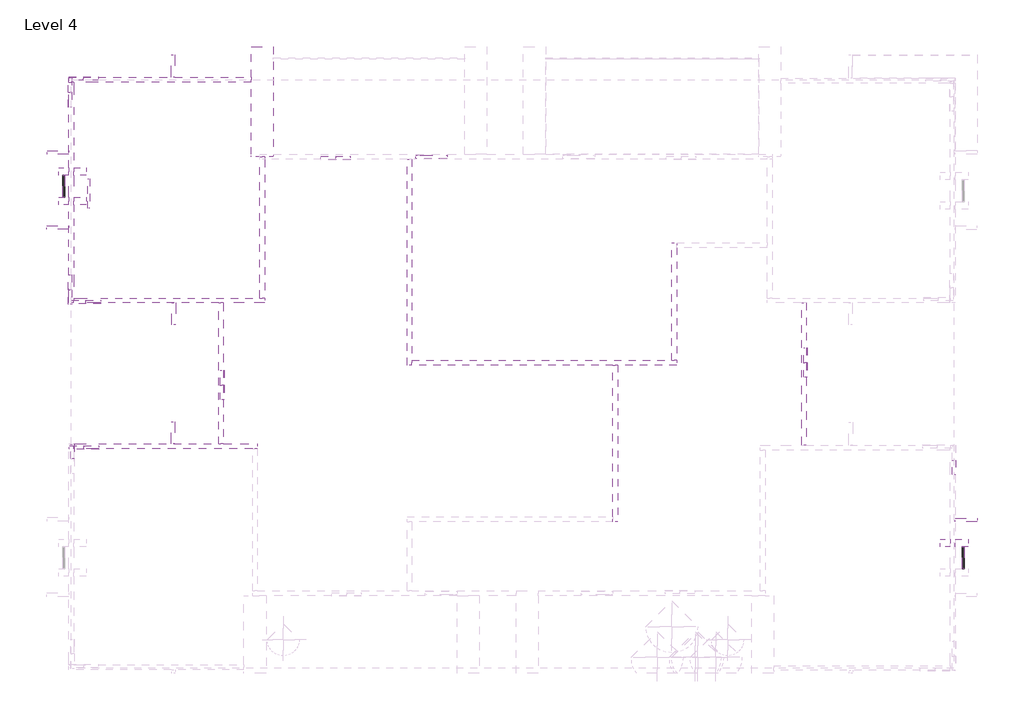
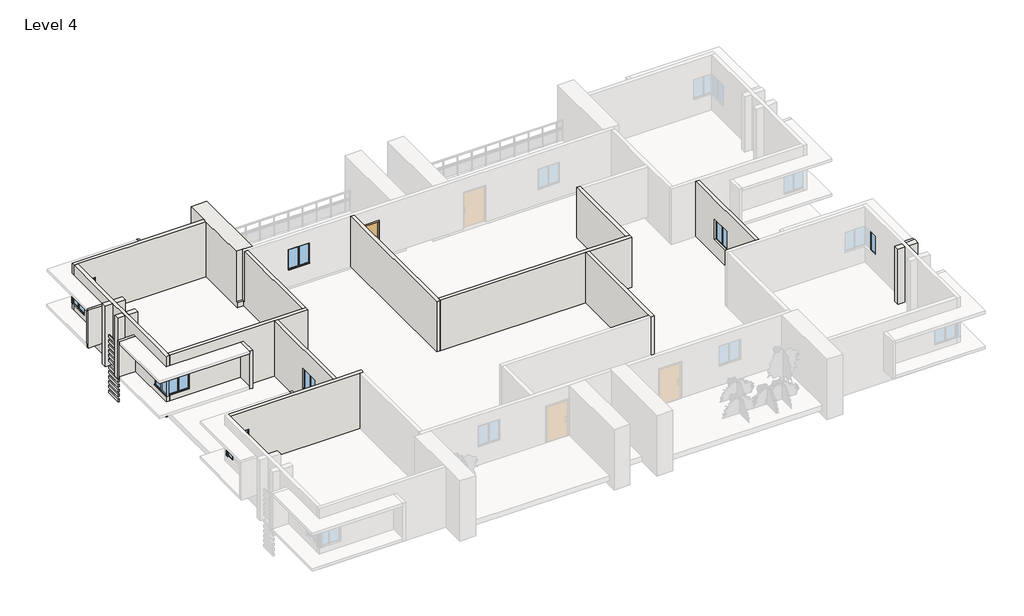
# One storey, part 2 of 4: 49 walls, 18 windows, 1 door.
"""IFC4 building model written with IfcOpenShell, lengths in millimetres."""

from ifc_helpers import new_model, si_unit, frame, origin, place, context, project, spatial, polyline, outline, extrude, faceted_brep, transform, mapped, element, save
from components import door_15d3c954, window_20ff4747

model = new_model("IFC4")

# Units and contexts
model_context = context("Model", 3, world=origin())
ifc_project = project(units=[si_unit("LENGTHUNIT", "METRE", prefix="MILLI")], contexts=[model_context])

# Site, building, storey
site = spatial("IfcSite", under=ifc_project)
building = spatial("IfcBuilding", under=site)
storey = spatial("IfcBuildingStorey", under=building, Name="Level 4", Elevation=9144.0)

# Door
placement = place(None, origin())
door_shape = door_15d3c954(model_context)
element("IfcDoor", 1, ObjectType="Door-Passage-Single-Flush-Dbl_Acting : 48\" x 96\"", at=placement, inside=storey, context=model_context, shape_type="MappedRepresentation", body=[
    mapped(door_shape, transform((153.0520665, 12804.5205944, 10972.8), x_axis=(1.0, 0.0, 0.0), y_axis=(0.0, 1.0, 0.0), z_axis=(0.0, 0.0, 1.0))),
])

# Walls
element("IfcWall", 2, ObjectType="Generic - 1'", at=placement, inside=storey, context=model_context, shape_type="SweptSolid", body=[
    extrude(outline(polyline([(-14151.7972154, 12048.8705944), (-14667.8479335, 12048.8705944), (-14667.8479335, 12353.6705944), (-14151.7972154, 12353.6705944), (-14151.7972154, 12048.8705944)])), frame((0.0, 0.0, 10363.2), z_axis=(0.0, 0.0, 1.0), x_axis=(1.0, 0.0, 0.0)), (0.0, 0.0, 1.0), 3657.6),
])
element("IfcWall", 3, ObjectType="Generic - 1'", at=placement, inside=storey, context=model_context, shape_type="SweptSolid", body=[
    extrude(outline(polyline([(-15302.1394029, 12353.6705944), (-14871.0479335, 12353.6705944), (-14871.0479335, 12048.8705944), (-15302.1394029, 12048.8705944), (-15302.1394029, 12353.6705944)])), frame((0.0, 0.0, 10363.2), z_axis=(0.0, 0.0, 1.0), x_axis=(1.0, 0.0, 0.0)), (0.0, 0.0, 1.0), 3657.6),
])
element("IfcWall", 4, ObjectType="Generic - 1'", at=placement, inside=storey, context=model_context, shape_type="SweptSolid", body=[
    extrude(outline(polyline([(-14151.7972154, 10829.6705944), (-14667.8479335, 10829.6705944), (-14667.8479335, 11134.4705944), (-14151.7972154, 11134.4705944), (-14151.7972154, 10829.6705944)])), frame((0.0, 0.0, 10363.2), z_axis=(0.0, 0.0, 1.0), x_axis=(1.0, 0.0, 0.0)), (0.0, 0.0, 1.0), 3657.6),
])
element("IfcWall", 5, ObjectType="Generic - 1'", at=placement, inside=storey, context=model_context, shape_type="SweptSolid", body=[
    extrude(outline(polyline([(-15302.1394029, 11134.4705944), (-14871.0479335, 11134.4705944), (-14871.0479335, 10829.6705944), (-15302.1394029, 10829.6705944), (-15302.1394029, 11134.4705944)])), frame((0.0, 0.0, 10363.2), z_axis=(0.0, 0.0, 1.0), x_axis=(1.0, 0.0, 0.0)), (0.0, 0.0, 1.0), 3657.6),
])
element("IfcWall", 6, ObjectType="Generic - 1'", at=placement, inside=storey, context=model_context, shape_type="SweptSolid", body=[
    extrude(outline(polyline([(22386.1027846, -3343.5294056), (21857.3520665, -3343.5294056), (21857.3520665, -3038.7294056), (22386.1027846, -3038.7294056), (22386.1027846, -3343.5294056)])), frame((0.0, 0.0, 10363.2), z_axis=(0.0, 0.0, 1.0), x_axis=(1.0, 0.0, 0.0)), (0.0, 0.0, 1.0), 3657.6),
])
element("IfcWall", 7, ObjectType="Generic - 1'", at=placement, inside=storey, context=model_context, shape_type="SweptSolid", body=[
    extrude(outline(polyline([(21235.7605971, -3038.7294056), (21654.1520665, -3038.7294056), (21654.1520665, -3343.5294056), (21235.7605971, -3343.5294056), (21235.7605971, -3038.7294056)])), frame((0.0, 0.0, 10363.2), z_axis=(0.0, 0.0, 1.0), x_axis=(1.0, 0.0, 0.0)), (0.0, 0.0, 1.0), 3657.6),
])
element("IfcWall", 8, ObjectType="Generic - 3'", at=placement, inside=storey, context=model_context, shape_type="Brep", body=[
    faceted_brep([(-6400.1479335, 12810.8705944, 10363.2), (-6400.1479335, 17382.8705944, 10363.2), (-6400.1479335, 17382.8705944, 14020.8), (-6400.1479335, 12912.4705944, 14020.8), (-6400.1479335, 12912.4705944, 10972.8), (-6400.1479335, 12810.8705944, 10972.8), (-7314.5479335, 12810.8705944, 10363.2), (-7314.5479335, 12810.8705944, 10972.8), (-7314.5479335, 12912.4705944, 10972.8), (-7314.5479335, 12912.4705944, 14020.8), (-7314.5479335, 15904.9548886, 14020.8), (-7314.5479335, 16108.1548886, 14020.8), (-7314.5479335, 17382.8705944, 14020.8), (-7314.5479335, 17382.8705944, 10363.2), (-7314.5479335, 16108.1548886, 10363.2), (-7314.5479335, 15904.9548886, 10363.2), (-6755.7479335, 12810.8705944, 10363.2), (-6958.9479335, 12810.8705944, 10363.2), (-6958.9479335, 12912.4705944, 14020.8), (-6755.7479335, 12810.8705944, 10972.8), (-6958.9479335, 12810.8705944, 10972.8), (-6958.9479335, 12912.4705944, 10972.8)], [[[0, 1, 2, 3, 4, 5]], [[6, 7, 8, 9, 10, 11, 12, 13, 14, 15]], [[1, 0, 16, 17, 6, 15, 14, 13]], [[2, 1, 13, 12]], [[3, 2, 12, 11, 10, 9, 18]], [[0, 5, 19, 20, 7, 6, 17, 16]], [[4, 21, 8, 7, 20, 19, 5]], [[4, 3, 18, 9, 8, 21]]]),
])
element("IfcWall", 9, ObjectType="Generic - 5\"", at=placement, inside=storey, context=model_context, shape_type="SweptSolid", body=[
    extrude(outline(polyline([(-15124.6936682, 11134.4705944), (-15124.6936682, 12048.8705944), (-15048.4936682, 12048.8705944), (-15048.4936682, 11134.4705944), (-15124.6936682, 11134.4705944)])), frame((0.0, 0.0, 8712.2), z_axis=(0.0, 0.0, 1.0), x_axis=(1.0, 0.0, 0.0)), (0.0, 0.0, 1.0), 152.8735856),
])
element("IfcWall", 10, ObjectType="Generic - 5\"", at=placement, inside=storey, context=model_context, shape_type="SweptSolid", body=[
    extrude(outline(polyline([(-15124.6936682, 11134.4705944), (-15124.6936682, 12048.8705944), (-15048.4936682, 12048.8705944), (-15048.4936682, 11134.4705944), (-15124.6936682, 11134.4705944)])), frame((0.0, 0.0, 9017.0), z_axis=(0.0, 0.0, 1.0), x_axis=(1.0, 0.0, 0.0)), (0.0, 0.0, 1.0), 152.8735856),
])
element("IfcWall", 11, ObjectType="Generic - 5\"", at=placement, inside=storey, context=model_context, shape_type="SweptSolid", body=[
    extrude(outline(polyline([(-15124.6936682, 11134.4705944), (-15124.6936682, 12048.8705944), (-15048.4936682, 12048.8705944), (-15048.4936682, 11134.4705944), (-15124.6936682, 11134.4705944)])), frame((0.0, 0.0, 9296.4), z_axis=(0.0, 0.0, 1.0), x_axis=(1.0, 0.0, 0.0)), (0.0, 0.0, 1.0), 152.8735856),
])
element("IfcWall", 12, ObjectType="Generic - 5\"", at=placement, inside=storey, context=model_context, shape_type="SweptSolid", body=[
    extrude(outline(polyline([(-15124.6936682, 11134.4705944), (-15124.6936682, 12048.8705944), (-15048.4936682, 12048.8705944), (-15048.4936682, 11134.4705944), (-15124.6936682, 11134.4705944)])), frame((0.0, 0.0, 9601.2), z_axis=(0.0, 0.0, 1.0), x_axis=(1.0, 0.0, 0.0)), (0.0, 0.0, 1.0), 152.8735856),
])
element("IfcWall", 13, ObjectType="Generic - 5\"", at=placement, inside=storey, context=model_context, shape_type="SweptSolid", body=[
    extrude(outline(polyline([(-15124.6936682, 11134.4705944), (-15124.6936682, 12048.8705944), (-15048.4936682, 12048.8705944), (-15048.4936682, 11134.4705944), (-15124.6936682, 11134.4705944)])), frame((0.0, 0.0, 9906.0), z_axis=(0.0, 0.0, 1.0), x_axis=(1.0, 0.0, 0.0)), (0.0, 0.0, 1.0), 152.8735856),
])
element("IfcWall", 14, ObjectType="Generic - 5\"", at=placement, inside=storey, context=model_context, shape_type="SweptSolid", body=[
    extrude(outline(polyline([(-15124.6936682, 11134.4705944), (-15124.6936682, 12048.8705944), (-15048.4936682, 12048.8705944), (-15048.4936682, 11134.4705944), (-15124.6936682, 11134.4705944)])), frame((0.0, 0.0, 10210.8), z_axis=(0.0, 0.0, 1.0), x_axis=(1.0, 0.0, 0.0)), (0.0, 0.0, 1.0), 152.8735856),
])
element("IfcWall", 15, ObjectType="Generic - 5\"", at=placement, inside=storey, context=model_context, shape_type="SweptSolid", body=[
    extrude(outline(polyline([(22145.9857703, -4257.9294056), (22145.9857703, -3343.5294056), (22222.1857703, -3343.5294056), (22222.1857703, -4257.9294056), (22145.9857703, -4257.9294056)])), frame((0.0, 0.0, 8712.2), z_axis=(0.0, 0.0, 1.0), x_axis=(1.0, 0.0, 0.0)), (0.0, 0.0, 1.0), 152.8735856),
])
element("IfcWall", 16, ObjectType="Generic - 5\"", at=placement, inside=storey, context=model_context, shape_type="SweptSolid", body=[
    extrude(outline(polyline([(22145.9857703, -4257.9294056), (22145.9857703, -3343.5294056), (22222.1857703, -3343.5294056), (22222.1857703, -4257.9294056), (22145.9857703, -4257.9294056)])), frame((0.0, 0.0, 9017.0), z_axis=(0.0, 0.0, 1.0), x_axis=(1.0, 0.0, 0.0)), (0.0, 0.0, 1.0), 152.8735856),
])
element("IfcWall", 17, ObjectType="Generic - 5\"", at=placement, inside=storey, context=model_context, shape_type="SweptSolid", body=[
    extrude(outline(polyline([(22145.9857703, -4257.9294056), (22145.9857703, -3343.5294056), (22222.1857703, -3343.5294056), (22222.1857703, -4257.9294056), (22145.9857703, -4257.9294056)])), frame((0.0, 0.0, 9296.4), z_axis=(0.0, 0.0, 1.0), x_axis=(1.0, 0.0, 0.0)), (0.0, 0.0, 1.0), 152.8735856),
])
element("IfcWall", 18, ObjectType="Generic - 5\"", at=placement, inside=storey, context=model_context, shape_type="SweptSolid", body=[
    extrude(outline(polyline([(22145.9857703, -4257.9294056), (22145.9857703, -3343.5294056), (22222.1857703, -3343.5294056), (22222.1857703, -4257.9294056), (22145.9857703, -4257.9294056)])), frame((0.0, 0.0, 9601.2), z_axis=(0.0, 0.0, 1.0), x_axis=(1.0, 0.0, 0.0)), (0.0, 0.0, 1.0), 152.8735856),
])
element("IfcWall", 19, ObjectType="Generic - 5\"", at=placement, inside=storey, context=model_context, shape_type="SweptSolid", body=[
    extrude(outline(polyline([(22145.9857703, -4257.9294056), (22145.9857703, -3343.5294056), (22222.1857703, -3343.5294056), (22222.1857703, -4257.9294056), (22145.9857703, -4257.9294056)])), frame((0.0, 0.0, 9906.0), z_axis=(0.0, 0.0, 1.0), x_axis=(1.0, 0.0, 0.0)), (0.0, 0.0, 1.0), 152.8735856),
])
element("IfcWall", 20, ObjectType="Generic - 5\"", at=placement, inside=storey, context=model_context, shape_type="SweptSolid", body=[
    extrude(outline(polyline([(22145.9857703, -4257.9294056), (22145.9857703, -3343.5294056), (22222.1857703, -3343.5294056), (22222.1857703, -4257.9294056), (22145.9857703, -4257.9294056)])), frame((0.0, 0.0, 10210.8), z_axis=(0.0, 0.0, 1.0), x_axis=(1.0, 0.0, 0.0)), (0.0, 0.0, 1.0), 152.8735856),
])
element("IfcWall", 21, ObjectType="Generic - 5\"", at=placement, inside=storey, context=model_context, shape_type="SweptSolid", body=[
    extrude(outline(polyline([(-15124.6936682, 11134.4705944), (-15124.6936682, 12048.8705944), (-15048.4936682, 12048.8705944), (-15048.4936682, 11134.4705944), (-15124.6936682, 11134.4705944)])), frame((0.0, 0.0, 10617.2), z_axis=(0.0, 0.0, 1.0), x_axis=(1.0, 0.0, 0.0)), (0.0, 0.0, 1.0), 152.8735856),
])
element("IfcWall", 22, ObjectType="Generic - 5\"", at=placement, inside=storey, context=model_context, shape_type="SweptSolid", body=[
    extrude(outline(polyline([(-14084.4224108, 10677.2705944), (-14084.4224108, 11896.4705944), (-14008.2224108, 11896.4705944), (-14008.2224108, 10677.2705944), (-14084.4224108, 10677.2705944)])), frame((0.0, 0.0, 10617.2), z_axis=(0.0, 0.0, 1.0), x_axis=(1.0, 0.0, 0.0)), (0.0, 0.0, 1.0), 178.1810075),
])
element("IfcWall", 23, ObjectType="Generic - 5\"", at=placement, inside=storey, context=model_context, shape_type="SweptSolid", body=[
    extrude(outline(polyline([(-15124.6936682, 11134.4705944), (-15124.6936682, 12048.8705944), (-15048.4936682, 12048.8705944), (-15048.4936682, 11134.4705944), (-15124.6936682, 11134.4705944)])), frame((0.0, 0.0, 10896.6), z_axis=(0.0, 0.0, 1.0), x_axis=(1.0, 0.0, 0.0)), (0.0, 0.0, 1.0), 152.8735856),
])
element("IfcWall", 24, ObjectType="Generic - 5\"", at=placement, inside=storey, context=model_context, shape_type="SweptSolid", body=[
    extrude(outline(polyline([(-15124.6936682, 11134.4705944), (-15124.6936682, 12048.8705944), (-15048.4936682, 12048.8705944), (-15048.4936682, 11134.4705944), (-15124.6936682, 11134.4705944)])), frame((0.0, 0.0, 11176.0), z_axis=(0.0, 0.0, 1.0), x_axis=(1.0, 0.0, 0.0)), (0.0, 0.0, 1.0), 152.8735856),
])
element("IfcWall", 25, ObjectType="Generic - 5\"", at=placement, inside=storey, context=model_context, shape_type="SweptSolid", body=[
    extrude(outline(polyline([(-15124.6936682, 11134.4705944), (-15124.6936682, 12048.8705944), (-15048.4936682, 12048.8705944), (-15048.4936682, 11134.4705944), (-15124.6936682, 11134.4705944)])), frame((0.0, 0.0, 11480.8), z_axis=(0.0, 0.0, 1.0), x_axis=(1.0, 0.0, 0.0)), (0.0, 0.0, 1.0), 152.8735856),
])
element("IfcWall", 26, ObjectType="Generic - 5\"", at=placement, inside=storey, context=model_context, shape_type="SweptSolid", body=[
    extrude(outline(polyline([(-15124.6936682, 11134.4705944), (-15124.6936682, 12048.8705944), (-15048.4936682, 12048.8705944), (-15048.4936682, 11134.4705944), (-15124.6936682, 11134.4705944)])), frame((0.0, 0.0, 11785.6), z_axis=(0.0, 0.0, 1.0), x_axis=(1.0, 0.0, 0.0)), (0.0, 0.0, 1.0), 152.8735856),
])
element("IfcWall", 27, ObjectType="Generic - 5\"", at=placement, inside=storey, context=model_context, shape_type="SweptSolid", body=[
    extrude(outline(polyline([(-15124.6936682, 11134.4705944), (-15124.6936682, 12048.8705944), (-15048.4936682, 12048.8705944), (-15048.4936682, 11134.4705944), (-15124.6936682, 11134.4705944)])), frame((0.0, 0.0, 12065.0), z_axis=(0.0, 0.0, 1.0), x_axis=(1.0, 0.0, 0.0)), (0.0, 0.0, 1.0), 152.8735856),
])
element("IfcWall", 28, ObjectType="Generic - 5\"", at=placement, inside=storey, context=model_context, shape_type="SweptSolid", body=[
    extrude(outline(polyline([(22145.9857703, -4257.9294056), (22145.9857703, -3343.5294056), (22222.1857703, -3343.5294056), (22222.1857703, -4257.9294056), (22145.9857703, -4257.9294056)])), frame((0.0, 0.0, 10617.2), z_axis=(0.0, 0.0, 1.0), x_axis=(1.0, 0.0, 0.0)), (0.0, 0.0, 1.0), 152.8735856),
])
element("IfcWall", 29, ObjectType="Generic - 5\"", at=placement, inside=storey, context=model_context, shape_type="SweptSolid", body=[
    extrude(outline(polyline([(22145.9857703, -4257.9294056), (22145.9857703, -3343.5294056), (22222.1857703, -3343.5294056), (22222.1857703, -4257.9294056), (22145.9857703, -4257.9294056)])), frame((0.0, 0.0, 10896.6), z_axis=(0.0, 0.0, 1.0), x_axis=(1.0, 0.0, 0.0)), (0.0, 0.0, 1.0), 152.8735856),
])
element("IfcWall", 30, ObjectType="Generic - 5\"", at=placement, inside=storey, context=model_context, shape_type="SweptSolid", body=[
    extrude(outline(polyline([(22145.9857703, -4257.9294056), (22145.9857703, -3343.5294056), (22222.1857703, -3343.5294056), (22222.1857703, -4257.9294056), (22145.9857703, -4257.9294056)])), frame((0.0, 0.0, 11176.0), z_axis=(0.0, 0.0, 1.0), x_axis=(1.0, 0.0, 0.0)), (0.0, 0.0, 1.0), 152.8735856),
])
element("IfcWall", 31, ObjectType="Generic - 5\"", at=placement, inside=storey, context=model_context, shape_type="SweptSolid", body=[
    extrude(outline(polyline([(22145.9857703, -4257.9294056), (22145.9857703, -3343.5294056), (22222.1857703, -3343.5294056), (22222.1857703, -4257.9294056), (22145.9857703, -4257.9294056)])), frame((0.0, 0.0, 11480.8), z_axis=(0.0, 0.0, 1.0), x_axis=(1.0, 0.0, 0.0)), (0.0, 0.0, 1.0), 152.8735856),
])
element("IfcWall", 32, ObjectType="Generic - 5\"", at=placement, inside=storey, context=model_context, shape_type="SweptSolid", body=[
    extrude(outline(polyline([(22145.9857703, -4257.9294056), (22145.9857703, -3343.5294056), (22222.1857703, -3343.5294056), (22222.1857703, -4257.9294056), (22145.9857703, -4257.9294056)])), frame((0.0, 0.0, 11785.6), z_axis=(0.0, 0.0, 1.0), x_axis=(1.0, 0.0, 0.0)), (0.0, 0.0, 1.0), 152.8735856),
])
element("IfcWall", 33, ObjectType="Generic - 5\"", at=placement, inside=storey, context=model_context, shape_type="SweptSolid", body=[
    extrude(outline(polyline([(22145.9857703, -4257.9294056), (22145.9857703, -3343.5294056), (22222.1857703, -3343.5294056), (22222.1857703, -4257.9294056), (22145.9857703, -4257.9294056)])), frame((0.0, 0.0, 12065.0), z_axis=(0.0, 0.0, 1.0), x_axis=(1.0, 0.0, 0.0)), (0.0, 0.0, 1.0), 152.8735856),
])
element("IfcWall", 34, ObjectType="Generic - 6\"", at=placement, inside=storey, context=model_context, shape_type="SweptSolid", body=[
    extrude(outline(polyline([(-10480.7034654, 17035.2548886), (-10480.7034654, 16120.8548886), (-10633.1034654, 16120.8548886), (-10633.1034654, 17035.2548886), (-10480.7034654, 17035.2548886)])), frame((0.0, 0.0, 11125.2), z_axis=(0.0, 0.0, 1.0), x_axis=(1.0, 0.0, 0.0)), (0.0, 0.0, 1.0), 2286.0),
])
element("IfcWall", 35, ObjectType="Generic - 6\"", at=placement, inside=storey, context=model_context, shape_type="SweptSolid", body=[
    extrude(outline(polyline([(-15775.8097154, 13072.8548886), (-14883.7479335, 13072.8548886), (-14883.7479335, 12920.4548886), (-15775.8097154, 12920.4548886), (-15775.8097154, 13072.8548886)])), frame((0.0, 0.0, 11125.2), z_axis=(0.0, 0.0, 1.0), x_axis=(1.0, 0.0, 0.0)), (0.0, 0.0, 1.0), 2286.0),
])
element("IfcWall", 36, ObjectType="Generic - 6\"", at=placement, inside=storey, context=model_context, shape_type="SweptSolid", body=[
    extrude(outline(polyline([(-10603.8479335, 5846.5548886), (-10603.8479335, 6760.9548886), (-10451.4479335, 6760.9548886), (-10451.4479335, 5846.5548886), (-10603.8479335, 5846.5548886)])), frame((0.0, 0.0, 11125.2), z_axis=(0.0, 0.0, 1.0), x_axis=(1.0, 0.0, 0.0)), (0.0, 0.0, 1.0), 2286.0),
])
element("IfcWall", 37, ObjectType="Generic - 6\"", at=placement, inside=storey, context=model_context, shape_type="SweptSolid", body=[
    extrude(outline(polyline([(-15798.1479335, 9961.3548886), (-14883.7479335, 9961.3548886), (-14883.7479335, 9808.9548886), (-15798.1479335, 9808.9548886), (-15798.1479335, 9961.3548886)])), frame((0.0, 0.0, 11125.2), z_axis=(0.0, 0.0, 1.0), x_axis=(1.0, 0.0, 0.0)), (0.0, 0.0, 1.0), 2286.0),
])
element("IfcWall", 38, ObjectType="Generic - 6\"", at=placement, inside=storey, context=model_context, shape_type="SweptSolid", body=[
    extrude(outline(polyline([(-10480.7034654, 1834.0395301), (-10480.7034654, 919.6395301), (-10633.1034654, 919.6395301), (-10633.1034654, 1834.0395301), (-10480.7034654, 1834.0395301)])), frame((0.0, 0.0, 11125.2), z_axis=(0.0, 0.0, 1.0), x_axis=(1.0, 0.0, 0.0)), (0.0, 0.0, 1.0), 2286.0),
])
element("IfcWall", 39, ObjectType="Generic - 6\"", at=placement, inside=storey, context=model_context, shape_type="SweptSolid", body=[
    extrude(outline(polyline([(22771.7520665, -2309.5899195), (21857.3520665, -2309.5899195), (21857.3520665, -2157.1899195), (22771.7520665, -2157.1899195), (22771.7520665, -2309.5899195)])), frame((0.0, 0.0, 11125.2), z_axis=(0.0, 0.0, 1.0), x_axis=(1.0, 0.0, 0.0)), (0.0, 0.0, 1.0), 2286.0),
])
element("IfcWall", 40, ObjectType="Generic - 8\"", at=placement, inside=storey, context=model_context, shape_type="Brep", body=[
    faceted_brep([(-862.9479335, 12709.2705944, 10972.8), (-862.9479335, 4174.8705944, 10972.8), (-862.9479335, 4174.8705944, 14020.8), (-862.9479335, 12709.2705944, 14020.8), (-659.7479335, 12709.2705944, 10972.8), (-659.7479335, 12709.2705944, 14020.8), (-659.7479335, 4378.0705944, 14020.8), (-659.7479335, 4174.8705944, 14020.8), (-659.7479335, 4174.8705944, 10972.8), (-659.7479335, 4378.0705944, 10972.8)], [[[0, 1, 2, 3]], [[4, 5, 6, 7, 8, 9]], [[1, 0, 4, 9, 8]], [[3, 2, 7, 6, 5]], [[0, 3, 5, 4]], [[2, 1, 8, 7]]]),
])
element("IfcWall", 41, ObjectType="Generic - 8\"", at=placement, inside=storey, context=model_context, shape_type="Brep", body=[
    faceted_brep([(-659.7479335, 4174.8705944, 10972.8), (7671.4520665, 4174.8705944, 10972.8), (7874.6520665, 4174.8705944, 10972.8), (10313.0520665, 4174.8705944, 10972.8), (10313.0520665, 4174.8705944, 14020.8), (7874.6520665, 4174.8705944, 14020.8), (7671.4520665, 4174.8705944, 14020.8), (-659.7479335, 4174.8705944, 14020.8), (-659.7479335, 4378.0705944, 10972.8), (-659.7479335, 4378.0705944, 14020.8), (10109.8520665, 4378.0705944, 14020.8), (10313.0520665, 4378.0705944, 14020.8), (10313.0520665, 4378.0705944, 10972.8), (10109.8520665, 4378.0705944, 10972.8)], [[[0, 1, 2, 3, 4, 5, 6, 7]], [[8, 9, 10, 11, 12, 13]], [[3, 2, 1, 0, 8, 13, 12]], [[7, 6, 5, 4, 11, 10, 9]], [[0, 7, 9, 8]], [[4, 3, 12, 11]]]),
])
element("IfcWall", 42, ObjectType="Generic - 8\"", at=placement, inside=storey, context=model_context, shape_type="Brep", body=[
    faceted_brep([(10313.0520665, 4378.0705944, 10972.8), (10313.0520665, 9051.6705944, 10972.8), (10313.0520665, 9254.8705944, 10972.8), (10313.0520665, 9254.8705944, 14020.8), (10313.0520665, 9051.6705944, 14020.8), (10313.0520665, 4378.0705944, 14020.8), (10109.8520665, 4378.0705944, 10972.8), (10109.8520665, 4378.0705944, 14020.8), (10109.8520665, 9254.8705944, 14020.8), (10109.8520665, 9254.8705944, 10972.8)], [[[0, 1, 2, 3, 4, 5]], [[6, 7, 8, 9]], [[2, 1, 0, 6, 9]], [[5, 4, 3, 8, 7]], [[0, 5, 7, 6]], [[3, 2, 9, 8]]]),
])
element("IfcWall", 43, ObjectType="Generic - 8\"", at=placement, inside=storey, context=model_context, shape_type="Brep", body=[
    faceted_brep([(7671.4520665, 4174.8705944, 10972.8), (7671.4520665, -2102.9604699, 10972.8), (7671.4520665, -2306.1604699, 10972.8), (7671.4520665, -2306.1604699, 14020.8), (7671.4520665, -2102.9604699, 14020.8), (7671.4520665, 4174.8705944, 14020.8), (7874.6520665, 4174.8705944, 10972.8), (7874.6520665, 4174.8705944, 14020.8), (7874.6520665, -2306.1604699, 14020.8), (7874.6520665, -2306.1604699, 10972.8)], [[[0, 1, 2, 3, 4, 5]], [[6, 7, 8, 9]], [[2, 1, 0, 6, 9]], [[5, 4, 3, 8, 7]], [[0, 5, 7, 6]], [[3, 2, 9, 8]]]),
])
element("IfcWall", 44, ObjectType="Generic - 8\" gray", at=placement, inside=storey, context=model_context, shape_type="Brep", body=[
    faceted_brep([(-14871.0479335, 15904.9548886, 10363.2), (-14667.8479335, 15904.9548886, 10363.2), (-7314.5479335, 15904.9548886, 10363.2), (-7314.5479335, 15904.9548886, 14020.8), (-14667.8479335, 15904.9548886, 14020.8), (-14871.0479335, 15904.9548886, 14020.8), (-14871.0479335, 15904.9548886, 12854.6804451), (-14667.8479335, 15904.9548886, 12854.6804451), (-13661.292575, 15904.9548886, 12854.6804451), (-13661.292575, 15904.9548886, 11635.4804451), (-14667.8479335, 15904.9548886, 11635.4804451), (-14871.0479335, 15904.9548886, 11635.4804451), (-7314.5479335, 16108.1548886, 10363.2), (-14871.0479335, 16108.1548886, 10363.2), (-14871.0479335, 16108.1548886, 11635.4804451), (-13661.292575, 16108.1548886, 11635.4804451), (-13661.292575, 16108.1548886, 12854.6804451), (-14871.0479335, 16108.1548886, 12854.6804451), (-14871.0479335, 16108.1548886, 14020.8), (-7314.5479335, 16108.1548886, 14020.8)], [[[0, 1, 2, 3, 4, 5, 6, 7, 8, 9, 10, 11]], [[12, 13, 14, 15, 16, 17, 18, 19]], [[2, 1, 0, 13, 12]], [[5, 4, 3, 19, 18]], [[5, 18, 17, 6]], [[13, 0, 11, 14]], [[3, 2, 12, 19]], [[9, 15, 14, 11, 10]], [[6, 17, 16, 8, 7]], [[8, 16, 15, 9]]]),
])
element("IfcWall", 45, ObjectType="Generic - 8\" gray", at=placement, inside=storey, context=model_context, shape_type="Brep", body=[
    faceted_brep([(-14667.8479335, 6760.9548886, 10363.2), (-14667.8479335, 6964.1548886, 10363.2), (-14667.8479335, 10829.6705944, 10363.2), (-14667.8479335, 11134.4705944, 10363.2), (-14667.8479335, 12048.8705944, 10363.2), (-14667.8479335, 12353.6705944, 10363.2), (-14667.8479335, 15904.9548886, 10363.2), (-14667.8479335, 15904.9548886, 11635.4804451), (-14667.8479335, 14871.0236266, 11635.4804451), (-14667.8479335, 14871.0236266, 12854.6804451), (-14667.8479335, 15904.9548886, 12854.6804451), (-14667.8479335, 15904.9548886, 14020.8), (-14667.8479335, 12353.6705944, 14020.8), (-14667.8479335, 12048.8705944, 14020.8), (-14667.8479335, 11134.4705944, 14020.8), (-14667.8479335, 10829.6705944, 14020.8), (-14667.8479335, 6964.1548886, 14020.8), (-14667.8479335, 6760.9548886, 14020.8), (-14667.8479335, 6760.9548886, 12854.6804451), (-14667.8479335, 6964.1548886, 12854.6804451), (-14667.8479335, 7918.4820466, 12854.6804451), (-14667.8479335, 7918.4820466, 11635.4804451), (-14667.8479335, 6964.1548886, 11635.4804451), (-14667.8479335, 6760.9548886, 11635.4804451), (-14871.0479335, 15904.9548886, 10363.2), (-14871.0479335, 12353.6705944, 10363.2), (-14871.0479335, 12048.8705944, 10363.2), (-14871.0479335, 11134.4705944, 10363.2), (-14871.0479335, 10829.6705944, 10363.2), (-14871.0479335, 6760.9548886, 10363.2), (-14871.0479335, 6760.9548886, 11635.4804451), (-14871.0479335, 7918.4820466, 11635.4804451), (-14871.0479335, 7918.4820466, 12854.6804451), (-14871.0479335, 6760.9548886, 12854.6804451), (-14871.0479335, 6760.9548886, 14020.8), (-14871.0479335, 10829.6705944, 14020.8), (-14871.0479335, 11134.4705944, 14020.8), (-14871.0479335, 12048.8705944, 14020.8), (-14871.0479335, 12353.6705944, 14020.8), (-14871.0479335, 15904.9548886, 14020.8), (-14871.0479335, 15904.9548886, 12854.6804451), (-14871.0479335, 14871.0236266, 12854.6804451), (-14871.0479335, 14871.0236266, 11635.4804451), (-14871.0479335, 15904.9548886, 11635.4804451)], [[[0, 1, 2, 3, 4, 5, 6, 7, 8, 9, 10, 11, 12, 13, 14, 15, 16, 17, 18, 19, 20, 21, 22, 23]], [[24, 25, 26, 27, 28, 29, 30, 31, 32, 33, 34, 35, 36, 37, 38, 39, 40, 41, 42, 43]], [[6, 5, 4, 3, 2, 1, 0, 29, 28, 27, 26, 25, 24]], [[17, 16, 15, 14, 13, 12, 11, 39, 38, 37, 36, 35, 34]], [[17, 34, 33, 18]], [[29, 0, 23, 30]], [[6, 24, 43, 7]], [[39, 11, 10, 40]], [[30, 23, 22, 21, 31]], [[18, 33, 32, 20, 19]], [[20, 32, 31, 21]], [[7, 43, 42, 8]], [[9, 8, 42, 41]], [[9, 41, 40, 10]]]),
])
element("IfcWall", 46, ObjectType="Generic - 8\" gray", at=placement, inside=storey, context=model_context, shape_type="Brep", body=[
    faceted_brep([(-6755.7479335, 6964.1548886, 10363.2), (-6958.9479335, 6964.1548886, 10363.2), (-14667.8479335, 6964.1548886, 10363.2), (-14667.8479335, 6964.1548886, 11635.4804451), (-13556.3228261, 6964.1548886, 11635.4804451), (-13556.3228261, 6964.1548886, 12854.6804451), (-14667.8479335, 6964.1548886, 12854.6804451), (-14667.8479335, 6964.1548886, 14020.8), (-6958.9479335, 6964.1548886, 14020.8), (-6755.7479335, 6964.1548886, 14020.8), (-14667.8479335, 6760.9548886, 10363.2), (-8673.4479335, 6760.9548886, 10363.2), (-8470.2479335, 6760.9548886, 10363.2), (-6755.7479335, 6760.9548886, 10363.2), (-6755.7479335, 6760.9548886, 14020.8), (-8470.2479335, 6760.9548886, 14020.8), (-8673.4479335, 6760.9548886, 14020.8), (-14667.8479335, 6760.9548886, 14020.8), (-14667.8479335, 6760.9548886, 12854.6804451), (-13556.3228261, 6760.9548886, 12854.6804451), (-13556.3228261, 6760.9548886, 11635.4804451), (-14667.8479335, 6760.9548886, 11635.4804451)], [[[0, 1, 2, 3, 4, 5, 6, 7, 8, 9]], [[10, 11, 12, 13, 14, 15, 16, 17, 18, 19, 20, 21]], [[2, 1, 0, 13, 12, 11, 10]], [[9, 8, 7, 17, 16, 15, 14]], [[2, 10, 21, 3]], [[17, 7, 6, 18]], [[0, 9, 14, 13]], [[3, 21, 20, 4]], [[5, 4, 20, 19]], [[5, 19, 18, 6]]]),
])
element("IfcWall", 47, ObjectType="Generic - 8\" gray", at=placement, inside=storey, context=model_context, shape_type="Brep", body=[
    faceted_brep([(-7060.5479335, 919.6395301, 10363.2), (-8470.2479335, 919.6395301, 10363.2), (-8673.4479335, 919.6395301, 10363.2), (-14680.5479335, 919.6395301, 10363.2), (-14680.5479335, 919.6395301, 11635.4804451), (-13641.9760869, 919.6395301, 11635.4804451), (-13641.9760869, 919.6395301, 12854.6804451), (-14680.5479335, 919.6395301, 12854.6804451), (-14680.5479335, 919.6395301, 14020.8), (-8673.4479335, 919.6395301, 14020.8), (-8470.2479335, 919.6395301, 14020.8), (-7060.5479335, 919.6395301, 14020.8), (-14680.5479335, 716.4395301, 10363.2), (-7263.7479335, 716.4395301, 10363.2), (-7060.5479335, 716.4395301, 10363.2), (-7060.5479335, 716.4395301, 14020.8), (-7263.7479335, 716.4395301, 14020.8), (-14680.5479335, 716.4395301, 14020.8), (-14680.5479335, 716.4395301, 12854.6804451), (-13641.9760869, 716.4395301, 12854.6804451), (-13641.9760869, 716.4395301, 11635.4804451), (-14680.5479335, 716.4395301, 11635.4804451), (-14680.5479335, 908.9135189, 11635.4804451), (-14680.5479335, 908.9135189, 12854.6804451)], [[[0, 1, 2, 3, 4, 5, 6, 7, 8, 9, 10, 11]], [[12, 13, 14, 15, 16, 17, 18, 19, 20, 21]], [[3, 2, 1, 0, 14, 13, 12]], [[11, 10, 9, 8, 17, 16, 15]], [[3, 12, 21, 22, 4]], [[17, 8, 7, 23, 18]], [[0, 11, 15, 14]], [[4, 22, 21, 20, 5]], [[6, 5, 20, 19]], [[6, 19, 18, 23, 7]]]),
])
element("IfcWall", 48, ObjectType="Generic - 8\" gray", at=placement, inside=storey, context=model_context, shape_type="SweptSolid", body=[
    extrude(outline(polyline([(6760.9548886, 10363.2), (919.6395301, 10363.2), (919.6395301, 14020.8), (6760.9548886, 14020.8), (6760.9548886, 10363.2)]), holes=[polyline([(2742.9076732, 11635.4804451), (3962.1076732, 11635.4804451), (3962.1076732, 12854.6804451), (2742.9076732, 12854.6804451), (2742.9076732, 11635.4804451)])]), frame((-8673.4479335, 0.0, 0.0), z_axis=(1.0, 0.0, 0.0), x_axis=(0.0, 1.0, 0.0)), (0.0, 0.0, 1.0), 203.2),
])
element("IfcWall", 49, ObjectType="Generic - 8\" gray", at=placement, inside=storey, context=model_context, shape_type="SweptSolid", body=[
    extrude(outline(polyline([(6760.9548886, 10363.2), (868.1548886, 10363.2), (868.1548886, 14020.8), (6760.9548886, 14020.8), (6760.9548886, 10363.2)]), holes=[polyline([(3676.3636585, 11635.4804451), (4895.5636585, 11635.4804451), (4895.5636585, 12854.6804451), (3676.3636585, 12854.6804451), (3676.3636585, 11635.4804451)])]), frame((15481.9520665, 0.0, 0.0), z_axis=(1.0, 0.0, 0.0), x_axis=(0.0, 1.0, 0.0)), (0.0, 0.0, 1.0), 203.2),
])
element("IfcWall", 50, ObjectType="Generic - 8\" gray", at=placement, inside=storey, context=model_context, shape_type="SweptSolid", body=[
    extrude(outline(polyline([(6964.1548886, 10363.2), (6964.1548886, 14020.8), (12709.2705944, 14020.8), (12709.2705944, 10972.8), (12810.8705944, 10972.8), (12810.8705944, 10363.2), (6964.1548886, 10363.2)])), frame((-6958.9479335, 0.0, 0.0), z_axis=(1.0, 0.0, 0.0), x_axis=(0.0, 1.0, 0.0)), (0.0, 0.0, 1.0), 203.2),
])

# Windows
window_shape = window_20ff4747(model_context)
element("IfcWindow", 51, ObjectType="Instance - Fixed : 24\" x 48\"", at=placement, inside=storey, context=model_context, shape_type="MappedRepresentation", body=[
    mapped(window_shape, transform((21755.7520665, -93.135515, 10721.0804451), x_axis=(0.0, -1.0, 0.0), y_axis=(1.0, 0.0, 0.0), z_axis=(0.0, 0.0, 1.0))),
])
element("IfcWindow", 52, ObjectType="Instance - Fixed : 24\" x 48\"", at=placement, inside=storey, context=model_context, shape_type="MappedRepresentation", body=[
    mapped(window_shape, transform((-14782.1479335, 566.0135189, 10721.0804451), x_axis=(0.0, -1.0, 0.0), y_axis=(1.0, 0.0, 0.0), z_axis=(0.0, 0.0, 1.0))),
])
element("IfcWindow", 53, ObjectType="Instance - Fixed : 24\" x 48\"", at=placement, inside=storey, context=model_context, shape_type="MappedRepresentation", body=[
    mapped(window_shape, transform((-14594.4760869, 818.0395301, 10721.0804451), x_axis=(-1.0, 0.0, 0.0), y_axis=(0.0, -1.0, 0.0), z_axis=(0.0, 0.0, 1.0))),
])
element("IfcWindow", 54, ObjectType="Instance - Fixed : 24\" x 48\"", at=placement, inside=storey, context=model_context, shape_type="MappedRepresentation", body=[
    mapped(window_shape, transform((-13984.8760869, 818.0395301, 10721.0804451), x_axis=(-1.0, 0.0, 0.0), y_axis=(0.0, -1.0, 0.0), z_axis=(0.0, 0.0, 1.0))),
])
element("IfcWindow", 55, ObjectType="Instance - Fixed : 24\" x 48\"", at=placement, inside=storey, context=model_context, shape_type="MappedRepresentation", body=[
    mapped(window_shape, transform((-14508.8228261, 6862.5548886, 10721.0804451), x_axis=(-1.0, 0.0, 0.0), y_axis=(0.0, -1.0, 0.0), z_axis=(0.0, 0.0, 1.0))),
])
element("IfcWindow", 56, ObjectType="Instance - Fixed : 24\" x 48\"", at=placement, inside=storey, context=model_context, shape_type="MappedRepresentation", body=[
    mapped(window_shape, transform((-13899.2228261, 6862.5548886, 10721.0804451), x_axis=(-1.0, 0.0, 0.0), y_axis=(0.0, -1.0, 0.0), z_axis=(0.0, 0.0, 1.0))),
])
element("IfcWindow", 57, ObjectType="Instance - Fixed : 24\" x 48\"", at=placement, inside=storey, context=model_context, shape_type="MappedRepresentation", body=[
    mapped(window_shape, transform((-14769.4479335, 7651.7820466, 10721.0804451), x_axis=(0.0, 1.0, 0.0), y_axis=(-1.0, 0.0, 0.0), z_axis=(0.0, 0.0, 1.0))),
])
element("IfcWindow", 58, ObjectType="Instance - Fixed : 24\" x 48\"", at=placement, inside=storey, context=model_context, shape_type="MappedRepresentation", body=[
    mapped(window_shape, transform((-14769.4479335, 7042.1820466, 10721.0804451), x_axis=(0.0, 1.0, 0.0), y_axis=(-1.0, 0.0, 0.0), z_axis=(0.0, 0.0, 1.0))),
])
element("IfcWindow", 59, ObjectType="Instance - Fixed : 24\" x 48\"", at=placement, inside=storey, context=model_context, shape_type="MappedRepresentation", body=[
    mapped(window_shape, transform((-14769.4479335, 15823.5236266, 10721.0804451), x_axis=(0.0, 1.0, 0.0), y_axis=(-1.0, 0.0, 0.0), z_axis=(0.0, 0.0, 1.0))),
])
element("IfcWindow", 60, ObjectType="Instance - Fixed : 24\" x 48\"", at=placement, inside=storey, context=model_context, shape_type="MappedRepresentation", body=[
    mapped(window_shape, transform((-14769.4479335, 15213.9236266, 10721.0804451), x_axis=(0.0, 1.0, 0.0), y_axis=(-1.0, 0.0, 0.0), z_axis=(0.0, 0.0, 1.0))),
])
element("IfcWindow", 61, ObjectType="Instance - Fixed : 24\" x 48\"", at=placement, inside=storey, context=model_context, shape_type="MappedRepresentation", body=[
    mapped(window_shape, transform((-13927.992575, 16006.5548886, 10721.0804451), x_axis=(1.0, 0.0, 0.0), y_axis=(0.0, 1.0, 0.0), z_axis=(0.0, 0.0, 1.0))),
])
element("IfcWindow", 62, ObjectType="Instance - Fixed : 24\" x 48\"", at=placement, inside=storey, context=model_context, shape_type="MappedRepresentation", body=[
    mapped(window_shape, transform((-14537.592575, 16006.5548886, 10721.0804451), x_axis=(1.0, 0.0, 0.0), y_axis=(0.0, 1.0, 0.0), z_axis=(0.0, 0.0, 1.0))),
])
element("IfcWindow", 63, ObjectType="Instance - Fixed : 24\" x 48\"", at=placement, inside=storey, context=model_context, shape_type="MappedRepresentation", body=[
    mapped(window_shape, transform((-4165.821881, 12810.8705944, 11103.8298362), x_axis=(-1.0, 0.0, 0.0), y_axis=(0.0, -1.0, 0.0), z_axis=(0.0, 0.0, 1.0))),
])
element("IfcWindow", 64, ObjectType="Instance - Fixed : 24\" x 48\"", at=placement, inside=storey, context=model_context, shape_type="MappedRepresentation", body=[
    mapped(window_shape, transform((-3556.221881, 12810.8705944, 11103.8298362), x_axis=(-1.0, 0.0, 0.0), y_axis=(0.0, -1.0, 0.0), z_axis=(0.0, 0.0, 1.0))),
])
element("IfcWindow", 65, ObjectType="Instance - Fixed : 24\" x 48\"", at=placement, inside=storey, context=model_context, shape_type="MappedRepresentation", body=[
    mapped(window_shape, transform((-8571.8479335, 3009.6076732, 10721.0804451), x_axis=(0.0, -1.0, 0.0), y_axis=(1.0, 0.0, 0.0), z_axis=(0.0, 0.0, 1.0))),
])
element("IfcWindow", 66, ObjectType="Instance - Fixed : 24\" x 48\"", at=placement, inside=storey, context=model_context, shape_type="MappedRepresentation", body=[
    mapped(window_shape, transform((-8571.8479335, 3619.2076732, 10721.0804451), x_axis=(0.0, -1.0, 0.0), y_axis=(1.0, 0.0, 0.0), z_axis=(0.0, 0.0, 1.0))),
])
element("IfcWindow", 67, ObjectType="Instance - Fixed : 24\" x 48\"", at=placement, inside=storey, context=model_context, shape_type="MappedRepresentation", body=[
    mapped(window_shape, transform((15583.5520665, 3943.0636585, 10721.0804451), x_axis=(0.0, -1.0, 0.0), y_axis=(1.0, 0.0, 0.0), z_axis=(0.0, 0.0, 1.0))),
])
element("IfcWindow", 68, ObjectType="Instance - Fixed : 24\" x 48\"", at=placement, inside=storey, context=model_context, shape_type="MappedRepresentation", body=[
    mapped(window_shape, transform((15583.5520665, 4552.6636585, 10721.0804451), x_axis=(0.0, -1.0, 0.0), y_axis=(1.0, 0.0, 0.0), z_axis=(0.0, 0.0, 1.0))),
])

save(model, "model.ifc")

# Revit data of these elements
# Type "Door-Passage-Single-Flush-Dbl_Acting : 48\" x 96\""
#   Type Mark = "12"
#   Assembly Code = "B2030200"
#   Analytic Construction = "Wooden"
#   Thickness = 0' - 1 3/4"
#   Thermal Resistance (R) = 2.5876 (h·ft²·°F)/BTU
#   Swing Angle [instance default] = 45.00°
#   Strike Height = 3' - 4"
#   Rough Width [instance default] = 4' - 4"
#   Rough Height [instance default] = 7' - 4"
#   MF Opening Height [instance default] = 0' - 4"
#   MF Opening Width [instance default] = 0' - 4"
#   Inset Calculate [instance default] = 0' - 4"
#   Masonry Inset [instance default] = 0' - 1"
#   Height = 7' - 0"
#   Width = 4' - 0"
#   Heat Transfer Coefficient (U) = 0.3865 BTU/(h·ft²·°F)
#   Masonry Frame Depth = 0' - 5 3/4"
#   Masonry Frame [instance default] = yes
#   Function = 1
#   Dry Wall Frame [instance default] = no
#   Panel Material = Wood - Birch
#   Frame Material = Metal - Paint Finish - Grey
#   Door Handle Material = Aluminum
#   Visual Light Transmittance = 0
#   Solar Heat Gain Coefficient = 0
#   Wall Closure = (empty or 0)
# Type "Generic - 1'"
#   Assembly Code = "B2010"
#   Layers, outside or top first: 1' - 0" "Metal - Painted - Grey" (function 1)
# Type "Generic - 3'"
#   Assembly Code = "B2010"
#   Layers, outside or top first: 3' - 0" "Metal - Painted - Grey" (function 1)
# Type "Generic - 5\""
#   Assembly Code = "B2010"
#   Layers, outside or top first: 0' - 3" "Oak Flooring" (function 1)
# Type "Generic - 6\""
#   Assembly Code = "B2010"
#   Layers, outside or top first: 0' - 6" "Metal - Painted - Grey" (function 1)
# Type "Generic - 8\""
#   Assembly Code = "B2010"
#   Layers, outside or top first: 0' - 8" no material (function 1)
# Type "Generic - 8\" gray"
#   Assembly Code = "B2010"
#   Layers, outside or top first: 0' - 8" "Parking Stripe" (function 1)
# Type "Instance - Fixed : 24\" x 48\""
#   Type Mark = "11"
#   Construction Type Id = "GSP4R"
#   Assembly Code = "B2020100"
#   Analytic Construction = "1/8 in Pilkington single glazing"
#   Visual Light Transmittance = 0.9
#   Thermal Resistance (R) = 0.8466 (h·ft²·°F)/BTU
#   Solar Heat Gain Coefficient = 0.86
#   Heat Transfer Coefficient (U) = 1.1812 BTU/(h·ft²·°F)
#   Height [instance default] = 4' - 0"
#   Default Sill Height = 3' - 0"
#   Width [instance default] = 2' - 0"
#   Window Inset = 0' - 2"
#   Define Thermal Properties by = 1
#   Glass Pane Material = Glass
#   Sash Material = Iron, Ductile
#   Wall Closure = (empty or 0)
# Element 1 (IfcDoor, "Door-Passage-Single-Flush-Dbl_Acting : 48\" x 96\"")
#   Swing Angle = 45.00°
#   Rough Width = 4' - 4"
#   Rough Height = 7' - 4"
#   Masonry Inset = 0' - 1"
#   MF Opening Width = 0' - 4"
#   MF Opening Height = 0' - 4"
#   Inset Calculate = 0' - 4"
#   Masonry Frame = yes
#   Dry Wall Frame = no
#   Phase Created = New Construction
#   Materials on its faces: "Aluminum", "Metal - Paint Finish - Grey", "Wood - Birch"
# Elements 2, 3, 4, 5, 6, 7 (IfcWall, "Generic - 1'")
#   built-in parameter 1001111 = 4' - 0"
#   Top Offset = 0' - 0"
#   Base Offset = 4' - 0"
#   Unconnected Height = 12' - 0"
#   wall height = 12' - 0"
#   Phase Created = New Construction
#   Base Constraint = Level 4
#   Materials on its faces: "Metal - Painted - Grey"
# Element 8 (IfcWall, "Generic - 3'")
#   built-in parameter 1001111 = 4' - 0"
#   Top Offset = 0' - 0"
#   Base Offset = 4' - 0"
#   Unconnected Height = 12' - 0"
#   wall height = 12' - 0"
#   Phase Created = New Construction
#   Base Constraint = Level 4
#   Materials on its faces: "Metal - Painted - Grey", "EIFS, Exterior Insulation"
# Elements 9, 15 (IfcWall, "Generic - 5\"")
#   built-in parameter 1001111 = -1' - 5"
#   Top Offset = -10' - 10.98135"
#   Base Offset = -1' - 5"
#   wall height = 0' - 6.01865"
#   Phase Created = New Construction
#   Base Constraint = Level 4
#   Top Constraint = Level 5
#   Materials on its faces: "Oak Flooring"
# Elements 10, 16 (IfcWall, "Generic - 5\"")
#   built-in parameter 1001111 = -0' - 5"
#   Top Offset = -9' - 10.98135"
#   Base Offset = -0' - 5"
#   wall height = 0' - 6.01865"
#   Phase Created = New Construction
#   Base Constraint = Level 4
#   Top Constraint = Level 5
#   Materials on its faces: "Oak Flooring"
# Elements 11, 17 (IfcWall, "Generic - 5\"")
#   built-in parameter 1001111 = 0' - 6"
#   Top Offset = -8' - 11.98135"
#   Base Offset = 0' - 6"
#   wall height = 0' - 6.01865"
#   Phase Created = New Construction
#   Base Constraint = Level 4
#   Top Constraint = Level 5
#   Materials on its faces: "Oak Flooring"
# Elements 12, 18 (IfcWall, "Generic - 5\"")
#   built-in parameter 1001111 = 1' - 6"
#   Top Offset = -7' - 11.98135"
#   Base Offset = 1' - 6"
#   wall height = 0' - 6.01865"
#   Phase Created = New Construction
#   Base Constraint = Level 4
#   Top Constraint = Level 5
#   Materials on its faces: "Oak Flooring"
# Elements 13, 19 (IfcWall, "Generic - 5\"")
#   built-in parameter 1001111 = 2' - 6"
#   Top Offset = -6' - 11.98135"
#   Base Offset = 2' - 6"
#   wall height = 0' - 6.01865"
#   Phase Created = New Construction
#   Base Constraint = Level 4
#   Top Constraint = Level 5
#   Materials on its faces: "Oak Flooring"
# Elements 14, 20 (IfcWall, "Generic - 5\"")
#   built-in parameter 1001111 = 3' - 6"
#   Top Offset = -5' - 11.98135"
#   Base Offset = 3' - 6"
#   wall height = 0' - 6.01865"
#   Phase Created = New Construction
#   Base Constraint = Level 4
#   Top Constraint = Level 5
#   Materials on its faces: "Oak Flooring"
# Elements 21, 28 (IfcWall, "Generic - 5\"")
#   built-in parameter 1001111 = 4' - 10"
#   Top Offset = -4' - 7.98135"
#   Base Offset = 4' - 10"
#   wall height = 0' - 6.01865"
#   Phase Created = New Construction
#   Base Constraint = Level 4
#   Top Constraint = Level 5
#   Materials on its faces: "Oak Flooring"
# Element 22 (IfcWall, "Generic - 5\"")
#   built-in parameter 1001111 = 4' - 10"
#   Top Offset = -4' - 6.985"
#   Base Offset = 4' - 10"
#   wall height = 0' - 7.015"
#   Phase Created = New Construction
#   Base Constraint = Level 4
#   Top Constraint = Level 5
#   Materials on its faces: "Oak Flooring"
# Elements 23, 29 (IfcWall, "Generic - 5\"")
#   built-in parameter 1001111 = 5' - 9"
#   Top Offset = -3' - 8.98135"
#   Base Offset = 5' - 9"
#   wall height = 0' - 6.01865"
#   Phase Created = New Construction
#   Base Constraint = Level 4
#   Top Constraint = Level 5
#   Materials on its faces: "Oak Flooring"
# Elements 24, 30 (IfcWall, "Generic - 5\"")
#   built-in parameter 1001111 = 6' - 8"
#   Top Offset = -2' - 9.98135"
#   Base Offset = 6' - 8"
#   wall height = 0' - 6.01865"
#   Phase Created = New Construction
#   Base Constraint = Level 4
#   Top Constraint = Level 5
#   Materials on its faces: "Oak Flooring"
# Elements 25, 31 (IfcWall, "Generic - 5\"")
#   built-in parameter 1001111 = 7' - 8"
#   Top Offset = -1' - 9.98135"
#   Base Offset = 7' - 8"
#   wall height = 0' - 6.01865"
#   Phase Created = New Construction
#   Base Constraint = Level 4
#   Top Constraint = Level 5
#   Materials on its faces: "Oak Flooring"
# Elements 26, 32 (IfcWall, "Generic - 5\"")
#   built-in parameter 1001111 = 8' - 8"
#   Top Offset = -0' - 9.98135"
#   Base Offset = 8' - 8"
#   wall height = 0' - 6.01865"
#   Phase Created = New Construction
#   Base Constraint = Level 4
#   Top Constraint = Level 5
#   Materials on its faces: "Oak Flooring"
# Elements 27, 33 (IfcWall, "Generic - 5\"")
#   built-in parameter 1001111 = 9' - 7"
#   Top Offset = 0' - 1.01865"
#   Base Offset = 9' - 7"
#   wall height = 0' - 6.01865"
#   Phase Created = New Construction
#   Base Constraint = Level 4
#   Top Constraint = Level 5
#   Materials on its faces: "Oak Flooring"
# Elements 34, 35, 36, 37, 38, 39 (IfcWall, "Generic - 6\"")
#   built-in parameter 1001111 = 6' - 6"
#   Top Offset = 0' - 0"
#   Base Offset = 6' - 6"
#   Unconnected Height = 7' - 6"
#   wall height = 7' - 6"
#   Phase Created = New Construction
#   Base Constraint = Level 4
#   Materials on its faces: "Metal - Painted - Grey"
# Elements 40, 41, 42, 43 (IfcWall, "Generic - 8\"")
#   built-in parameter 1001111 = 6' - 0"
#   Top Offset = 0' - 0"
#   Base Offset = 6' - 0"
#   Unconnected Height = 10' - 0"
#   wall height = 10' - 0"
#   Phase Created = New Construction
#   Base Constraint = Level 4
#   Materials on its faces: "Default Wall"
# Elements 44, 45, 46, 47, 48, 49, 50 (IfcWall, "Generic - 8\" gray")
#   built-in parameter 1001111 = 4' - 0"
#   Top Offset = 0' - 0"
#   Base Offset = 4' - 0"
#   Unconnected Height = 12' - 0"
#   wall height = 12' - 0"
#   Phase Created = New Construction
#   Base Constraint = Level 4
#   Materials on its faces: "Parking Stripe"
# Element 51 (IfcWindow, "Instance - Fixed : 24\" x 48\"")
#   Mark = "97"
#   Width = 2' - 0"
#   Height = 4' - 0"
#   Phase Created = New Construction
#   Materials on its faces: "Iron, Ductile", "Glass"
# Element 52 (IfcWindow, "Instance - Fixed : 24\" x 48\"")
#   Mark = "108"
#   Width = 2' - 0"
#   Height = 4' - 0"
#   Phase Created = New Construction
#   Materials on its faces: "Iron, Ductile", "Glass"
# Element 53 (IfcWindow, "Instance - Fixed : 24\" x 48\"")
#   Mark = "109"
#   Width = 2' - 0"
#   Height = 4' - 0"
#   Phase Created = New Construction
#   Materials on its faces: "Iron, Ductile", "Glass"
# Element 54 (IfcWindow, "Instance - Fixed : 24\" x 48\"")
#   Mark = "110"
#   Width = 2' - 0"
#   Height = 4' - 0"
#   Phase Created = New Construction
#   Materials on its faces: "Iron, Ductile", "Glass"
# Element 55 (IfcWindow, "Instance - Fixed : 24\" x 48\"")
#   Mark = "111"
#   Width = 2' - 0"
#   Height = 4' - 0"
#   Phase Created = New Construction
#   Materials on its faces: "Iron, Ductile", "Glass"
# Element 56 (IfcWindow, "Instance - Fixed : 24\" x 48\"")
#   Mark = "112"
#   Width = 2' - 0"
#   Height = 4' - 0"
#   Phase Created = New Construction
#   Materials on its faces: "Iron, Ductile", "Glass"
# Element 57 (IfcWindow, "Instance - Fixed : 24\" x 48\"")
#   Mark = "113"
#   Width = 2' - 0"
#   Height = 4' - 0"
#   Phase Created = New Construction
#   Materials on its faces: "Iron, Ductile", "Glass"
# Element 58 (IfcWindow, "Instance - Fixed : 24\" x 48\"")
#   Mark = "114"
#   Width = 2' - 0"
#   Height = 4' - 0"
#   Phase Created = New Construction
#   Materials on its faces: "Iron, Ductile", "Glass"
# Element 59 (IfcWindow, "Instance - Fixed : 24\" x 48\"")
#   Mark = "115"
#   Width = 2' - 0"
#   Height = 4' - 0"
#   Phase Created = New Construction
#   Materials on its faces: "Iron, Ductile", "Glass"
# Element 60 (IfcWindow, "Instance - Fixed : 24\" x 48\"")
#   Mark = "116"
#   Width = 2' - 0"
#   Height = 4' - 0"
#   Phase Created = New Construction
#   Materials on its faces: "Iron, Ductile", "Glass"
# Element 61 (IfcWindow, "Instance - Fixed : 24\" x 48\"")
#   Mark = "117"
#   Width = 2' - 0"
#   Height = 4' - 0"
#   Phase Created = New Construction
#   Materials on its faces: "Iron, Ductile", "Glass"
# Element 62 (IfcWindow, "Instance - Fixed : 24\" x 48\"")
#   Mark = "118"
#   Width = 2' - 0"
#   Height = 4' - 0"
#   Phase Created = New Construction
#   Materials on its faces: "Iron, Ductile", "Glass"
# Element 63 (IfcWindow, "Instance - Fixed : 24\" x 48\"")
#   Mark = "125"
#   Width = 2' - 0"
#   Height = 4' - 0"
#   Phase Created = New Construction
#   Materials on its faces: "Iron, Ductile", "Glass"
# Element 64 (IfcWindow, "Instance - Fixed : 24\" x 48\"")
#   Mark = "126"
#   Width = 2' - 0"
#   Height = 4' - 0"
#   Phase Created = New Construction
#   Materials on its faces: "Iron, Ductile", "Glass"
# Element 65 (IfcWindow, "Instance - Fixed : 24\" x 48\"")
#   Mark = "127"
#   Width = 2' - 0"
#   Height = 4' - 0"
#   Phase Created = New Construction
#   Materials on its faces: "Iron, Ductile", "Glass"
# Element 66 (IfcWindow, "Instance - Fixed : 24\" x 48\"")
#   Mark = "128"
#   Width = 2' - 0"
#   Height = 4' - 0"
#   Phase Created = New Construction
#   Materials on its faces: "Iron, Ductile", "Glass"
# Element 67 (IfcWindow, "Instance - Fixed : 24\" x 48\"")
#   Mark = "133"
#   Width = 2' - 0"
#   Height = 4' - 0"
#   Phase Created = New Construction
#   Materials on its faces: "Iron, Ductile", "Glass"
# Element 68 (IfcWindow, "Instance - Fixed : 24\" x 48\"")
#   Mark = "134"
#   Width = 2' - 0"
#   Height = 4' - 0"
#   Phase Created = New Construction
#   Materials on its faces: "Iron, Ductile", "Glass"
# Materials
#   "Wood - Birch": class "Wood", colour RGB 166 116 52, transparency 0, Cost = 0
#   "Metal - Paint Finish - Grey": class "Paint", colour RGB 104 104 104, transparency 0, Cost = 0
#   "Aluminum": class "Metal", colour RGB 247 247 247, transparency 0, Description = "Aluminum 6061", Cost = 0
#   "Metal - Painted - Grey": class "Paint", colour RGB 104 104 104, transparency 0, Cost = 0
#   "Oak Flooring": class "Wood", colour RGB 216 169 114, transparency 0, Description = "Quercus Rubra", Cost = 0
#   "Parking Stripe": class "Paint", colour RGB 250 250 91, transparency 0, Cost = 0
#   "Glass": class "Glass", colour RGB 0 128 192, transparency 0.75, Description = "Soda Lime Glass", Cost = 0
#   "Iron, Ductile": class "Metal", colour RGB 0 0 0, transparency 0, Description = "Ductile cast iron", Cost = 0
#   "EIFS, Exterior Insulation": class "Generic", colour RGB 127 127 127, transparency 0, Description = "EIFS - Exterior Insulation", Cost = 0
#   "Default Wall": colour RGB 128 128 128, transparency 0
